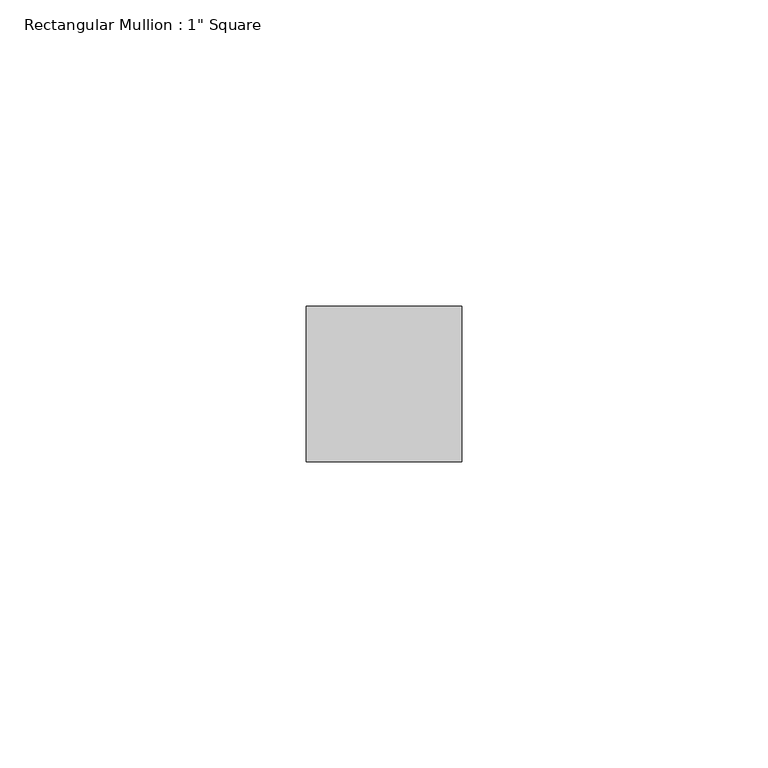
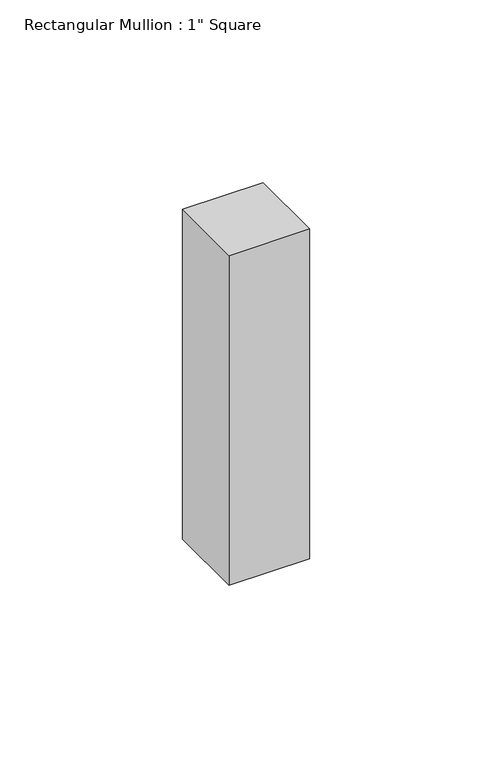
"""IFC4 building model written with IfcOpenShell, lengths in millimetres: member geometry."""

from ifc_helpers import new_model, si_unit, frame, origin, place, context, project, spatial, polyline, outline, extrude, source, transform, mapped, element, save


def member_fc53d4cb(model_context):
    return source(origin(), model_context, "Body", "SweptSolid", [
        extrude(outline(polyline([(0.0, 12.7), (0.0, -12.7), (-25.4, -12.7), (-25.4, 12.7), (0.0, 12.7)])), frame((0.0, 0.0, -110.0666667), z_axis=(0.0, 0.0, 1.0), x_axis=(1.0, 0.0, 0.0)), (0.0, 0.0, 1.0), 110.0666667),
    ])


if __name__ == "__main__":
    model = new_model("IFC4")
    model_context = context("Model", 3, world=origin())
    ifc_project = project(units=[si_unit("LENGTHUNIT", "METRE", prefix="MILLI")], contexts=[model_context])
    site = spatial("IfcSite", under=ifc_project)
    building = spatial("IfcBuilding", under=site)
    placement = place(None, origin())
    member_shape = member_fc53d4cb(model_context)
    element("IfcMember", 1, ObjectType="Rectangular Mullion : 1\" Square", at=placement, inside=building, context=model_context, shape_type="MappedRepresentation", body=[
        mapped(member_shape, transform((0.0, 0.0, 0.0), x_axis=(1.0, 0.0, 0.0), y_axis=(0.0, 1.0, 0.0), z_axis=(0.0, 0.0, 1.0))),
    ])
    save(model, "model.ifc")

# Revit data of these elements
# Type "Rectangular Mullion : 1\" Square"
#   built-in parameter 1007304 = 0.0833333 (stored number, unit not read)
#   built-in parameter 1007301 = 0.0416667 (stored number, unit not read)
#   built-in parameter 1007300 = 0.0416667 (stored number, unit not read)
# Element 1 (IfcMember, "Rectangular Mullion : 1\" Square")
#   Materials on its faces: "black"
# Materials
#   "black": class "Generic", colour RGB 120 120 120, transparency 0, Cost = 0
